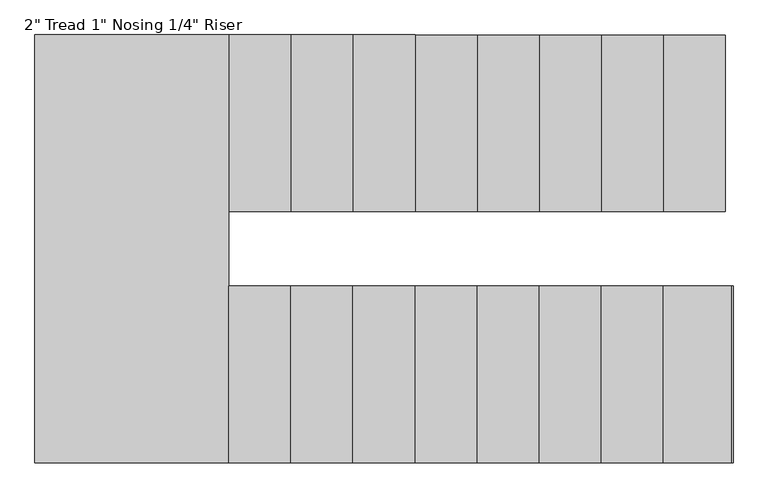
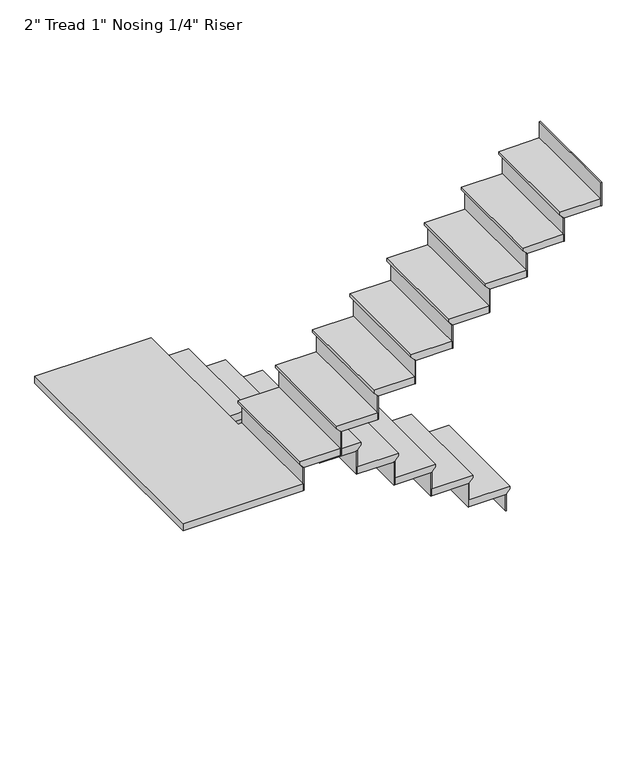
"""IFC4 building model written with IfcOpenShell, lengths in millimetres: stair flight geometry."""

from ifc_helpers import new_model, si_unit, origin, place, context, project, spatial, faceted_brep, source, transform, mapped, element, save


def stair_flight_4533c53f(model_context):
    return source(origin(), model_context, "Body", "Brep", [
        faceted_brep([(-2118.1728655, 1192.5797121, 148.8722222), (-2118.1728655, 1192.5797121, 167.9222222), (-2118.1728655, 468.6797121, 167.9222222), (-2118.1728655, 468.6797121, 148.8722222), (-2143.5728655, 1192.5797121, 123.4722222), (-2143.5728655, 468.6797121, 123.4722222), (-2397.5728655, 1192.5797121, 167.9222222), (-2397.5728655, 468.6797121, 167.9222222), (-2143.5728655, 468.6797121, 117.1222222), (-2397.5728655, 468.6797121, 117.1222222), (-2397.5728655, 1192.5797121, 117.1222222), (-2143.5728655, 1192.5797121, 117.1222222)], [[[0, 1, 2, 3]], [[4, 0, 3, 5]], [[2, 1, 6, 7]], [[8, 9, 10, 11]], [[2, 7, 9, 8, 5, 3]], [[8, 11, 4, 5]], [[6, 1, 0, 4, 11, 10]], [[7, 6, 10, 9]]]),
        faceted_brep([(-2143.5728655, 1192.5797121, 117.1222222), (-2143.5728655, 1192.5797121, 0.0), (-2149.9228655, 1192.5797121, 0.0), (-2149.9228655, 1192.5797121, 117.1222222), (-2143.5728655, 468.6797121, 117.1222222), (-2149.9228655, 468.6797121, 117.1222222), (-2149.9228655, 468.6797121, 0.0), (-2143.5728655, 468.6797121, 0.0)], [[[0, 1, 2, 3]], [[4, 5, 6, 7]], [[1, 0, 4, 7]], [[2, 1, 7, 6]], [[3, 2, 6, 5]], [[0, 3, 5, 4]]]),
        faceted_brep([(-2397.5728655, 1192.5797121, 285.0444444), (-2397.5728655, 1192.5797121, 117.1222222), (-2403.9228655, 1192.5797121, 117.1222222), (-2403.9228655, 1192.5797121, 285.0444444), (-2397.5728655, 468.6797121, 285.0444444), (-2403.9228655, 468.6797121, 285.0444444), (-2403.9228655, 468.6797121, 117.1222222), (-2397.5728655, 468.6797121, 117.1222222)], [[[0, 1, 2, 3]], [[4, 5, 6, 7]], [[1, 0, 4, 7]], [[2, 1, 7, 6]], [[3, 2, 6, 5]], [[0, 3, 5, 4]]]),
        faceted_brep([(-2372.1728655, 468.6797121, 335.8444444), (-2372.1728655, 1192.5797121, 335.8444444), (-2651.5728655, 1192.5797121, 335.8444444), (-2651.5728655, 468.6797121, 335.8444444), (-2397.5728655, 468.6797121, 285.0444444), (-2651.5728655, 468.6797121, 285.0444444), (-2651.5728655, 1192.5797121, 285.0444444), (-2397.5728655, 1192.5797121, 285.0444444), (-2397.5728655, 468.6797121, 291.3944444), (-2372.1728655, 468.6797121, 316.7944444), (-2397.5728655, 1192.5797121, 291.3944444), (-2372.1728655, 1192.5797121, 316.7944444)], [[[0, 1, 2, 3]], [[4, 5, 6, 7]], [[0, 3, 5, 4, 8, 9]], [[4, 7, 10, 8]], [[2, 1, 11, 10, 7, 6]], [[3, 2, 6, 5]], [[11, 1, 0, 9]], [[10, 11, 9, 8]]]),
        faceted_brep([(-2651.5728655, 1192.5797121, 452.9666667), (-2651.5728655, 1192.5797121, 285.0444444), (-2657.9228655, 1192.5797121, 285.0444444), (-2657.9228655, 1192.5797121, 452.9666667), (-2651.5728655, 468.6797121, 452.9666667), (-2657.9228655, 468.6797121, 452.9666667), (-2657.9228655, 468.6797121, 285.0444444), (-2651.5728655, 468.6797121, 285.0444444)], [[[0, 1, 2, 3]], [[4, 5, 6, 7]], [[1, 0, 4, 7]], [[2, 1, 7, 6]], [[3, 2, 6, 5]], [[0, 3, 5, 4]]]),
        faceted_brep([(-2626.1728655, 468.6797121, 503.7666667), (-2626.1728655, 1192.5797121, 503.7666667), (-2905.5728655, 1192.5797121, 503.7666667), (-2905.5728655, 468.6797121, 503.7666667), (-2651.5728655, 468.6797121, 452.9666667), (-2905.5728655, 468.6797121, 452.9666667), (-2905.5728655, 1192.5797121, 452.9666667), (-2651.5728655, 1192.5797121, 452.9666667), (-2651.5728655, 468.6797121, 459.3166667), (-2626.1728655, 468.6797121, 484.7166667), (-2651.5728655, 1192.5797121, 459.3166667), (-2626.1728655, 1192.5797121, 484.7166667)], [[[0, 1, 2, 3]], [[4, 5, 6, 7]], [[0, 3, 5, 4, 8, 9]], [[4, 7, 10, 8]], [[2, 1, 11, 10, 7, 6]], [[3, 2, 6, 5]], [[11, 1, 0, 9]], [[10, 11, 9, 8]]]),
        faceted_brep([(-2905.5728655, 1192.5797121, 620.8888889), (-2905.5728655, 1192.5797121, 452.9666667), (-2911.9228655, 1192.5797121, 452.9666667), (-2911.9228655, 1192.5797121, 620.8888889), (-2905.5728655, 468.6797121, 620.8888889), (-2911.9228655, 468.6797121, 620.8888889), (-2911.9228655, 468.6797121, 452.9666667), (-2905.5728655, 468.6797121, 452.9666667)], [[[0, 1, 2, 3]], [[4, 5, 6, 7]], [[1, 0, 4, 7]], [[2, 1, 7, 6]], [[3, 2, 6, 5]], [[0, 3, 5, 4]]]),
        faceted_brep([(-2880.1728655, 468.6797121, 671.6888889), (-2880.1728655, 1192.5797121, 671.6888889), (-3159.5728655, 1192.5797121, 671.6888889), (-3159.5728655, 468.6797121, 671.6888889), (-2905.5728655, 468.6797121, 620.8888889), (-3159.5728655, 468.6797121, 620.8888889), (-3159.5728655, 1192.5797121, 620.8888889), (-2905.5728655, 1192.5797121, 620.8888889), (-2905.5728655, 468.6797121, 627.2388889), (-2880.1728655, 468.6797121, 652.6388889), (-2905.5728655, 1192.5797121, 627.2388889), (-2880.1728655, 1192.5797121, 652.6388889)], [[[0, 1, 2, 3]], [[4, 5, 6, 7]], [[0, 3, 5, 4, 8, 9]], [[4, 7, 10, 8]], [[2, 1, 11, 10, 7, 6]], [[3, 2, 6, 5]], [[11, 1, 0, 9]], [[10, 11, 9, 8]]]),
        faceted_brep([(-3159.5728655, 1192.5797121, 788.8111111), (-3159.5728655, 1192.5797121, 620.8888889), (-3165.9228655, 1192.5797121, 620.8888889), (-3165.9228655, 1192.5797121, 788.8111111), (-3159.5728655, 468.6797121, 788.8111111), (-3165.9228655, 468.6797121, 788.8111111), (-3165.9228655, 468.6797121, 620.8888889), (-3159.5728655, 468.6797121, 620.8888889)], [[[0, 1, 2, 3]], [[4, 5, 6, 7]], [[1, 0, 4, 7]], [[2, 1, 7, 6]], [[3, 2, 6, 5]], [[0, 3, 5, 4]]]),
        faceted_brep([(-3134.1728655, 468.6797121, 839.6111111), (-3134.1728655, 1192.5797121, 839.6111111), (-3413.5728655, 1192.5797121, 839.6111111), (-3413.5728655, 468.6797121, 839.6111111), (-3159.5728655, 468.6797121, 788.8111111), (-3413.5728655, 468.6797121, 788.8111111), (-3413.5728655, 1192.5797121, 788.8111111), (-3159.5728655, 1192.5797121, 788.8111111), (-3159.5728655, 468.6797121, 795.1611111), (-3134.1728655, 468.6797121, 820.5611111), (-3159.5728655, 1192.5797121, 795.1611111), (-3134.1728655, 1192.5797121, 820.5611111)], [[[0, 1, 2, 3]], [[4, 5, 6, 7]], [[0, 3, 5, 4, 8, 9]], [[4, 7, 10, 8]], [[2, 1, 11, 10, 7, 6]], [[3, 2, 6, 5]], [[11, 1, 0, 9]], [[10, 11, 9, 8]]]),
        faceted_brep([(-3413.5728655, 1192.5797121, 956.7333333), (-3413.5728655, 1192.5797121, 788.8111111), (-3419.9228655, 1192.5797121, 788.8111111), (-3419.9228655, 1192.5797121, 956.7333333), (-3413.5728655, 468.6797121, 956.7333333), (-3419.9228655, 468.6797121, 956.7333333), (-3419.9228655, 468.6797121, 788.8111111), (-3413.5728655, 468.6797121, 788.8111111)], [[[0, 1, 2, 3]], [[4, 5, 6, 7]], [[1, 0, 4, 7]], [[2, 1, 7, 6]], [[3, 2, 6, 5]], [[0, 3, 5, 4]]]),
        faceted_brep([(-3388.1728655, 468.6797121, 1007.5333333), (-3388.1728655, 1192.5797121, 1007.5333333), (-3667.5728655, 1192.5797121, 1007.5333333), (-3667.5728655, 468.6797121, 1007.5333333), (-3413.5728655, 468.6797121, 956.7333333), (-3667.5728655, 468.6797121, 956.7333333), (-3667.5728655, 1192.5797121, 956.7333333), (-3413.5728655, 1192.5797121, 956.7333333), (-3413.5728655, 468.6797121, 963.0833333), (-3388.1728655, 468.6797121, 988.4833333), (-3413.5728655, 1192.5797121, 963.0833333), (-3388.1728655, 1192.5797121, 988.4833333)], [[[0, 1, 2, 3]], [[4, 5, 6, 7]], [[0, 3, 5, 4, 8, 9]], [[4, 7, 10, 8]], [[2, 1, 11, 10, 7, 6]], [[3, 2, 6, 5]], [[11, 1, 0, 9]], [[10, 11, 9, 8]]]),
        faceted_brep([(-3667.5728655, 1192.5797121, 1124.6555556), (-3667.5728655, 1192.5797121, 956.7333333), (-3673.9228655, 1192.5797121, 956.7333333), (-3673.9228655, 1192.5797121, 1124.6555556), (-3667.5728655, 468.6797121, 1124.6555556), (-3673.9228655, 468.6797121, 1124.6555556), (-3673.9228655, 468.6797121, 956.7333333), (-3667.5728655, 468.6797121, 956.7333333)], [[[0, 1, 2, 3]], [[4, 5, 6, 7]], [[1, 0, 4, 7]], [[2, 1, 7, 6]], [[3, 2, 6, 5]], [[0, 3, 5, 4]]]),
        faceted_brep([(-3642.1728655, 468.6797121, 1175.4555556), (-3642.1728655, 1192.5797121, 1175.4555556), (-3921.5728655, 1192.5797121, 1175.4555556), (-3921.5728655, 468.6797121, 1175.4555556), (-3667.5728655, 468.6797121, 1124.6555556), (-3921.5728655, 468.6797121, 1124.6555556), (-3921.5728655, 1192.5797121, 1124.6555556), (-3667.5728655, 1192.5797121, 1124.6555556), (-3667.5728655, 468.6797121, 1131.0055556), (-3642.1728655, 468.6797121, 1156.4055556), (-3667.5728655, 1192.5797121, 1131.0055556), (-3642.1728655, 1192.5797121, 1156.4055556)], [[[0, 1, 2, 3]], [[4, 5, 6, 7]], [[0, 3, 5, 4, 8, 9]], [[4, 7, 10, 8]], [[2, 1, 11, 10, 7, 6]], [[3, 2, 6, 5]], [[11, 1, 0, 9]], [[10, 11, 9, 8]]]),
        faceted_brep([(-3921.5728655, 1192.5797121, 1292.5777778), (-3921.5728655, 1192.5797121, 1124.6555556), (-3927.9228655, 1192.5797121, 1124.6555556), (-3927.9228655, 1192.5797121, 1292.5777778), (-3921.5728655, 468.6797121, 1292.5777778), (-3927.9228655, 468.6797121, 1292.5777778), (-3927.9228655, 468.6797121, 1124.6555556), (-3921.5728655, 468.6797121, 1124.6555556)], [[[0, 1, 2, 3]], [[4, 5, 6, 7]], [[1, 0, 4, 7]], [[2, 1, 7, 6]], [[3, 2, 6, 5]], [[0, 3, 5, 4]]]),
        faceted_brep([(-3896.1728655, 468.6797121, 1343.3777778), (-3896.1728655, 1192.5797121, 1343.3777778), (-4175.5728655, 1192.5797121, 1343.3777778), (-4175.5728655, 468.6797121, 1343.3777778), (-3921.5728655, 468.6797121, 1292.5777778), (-4175.5728655, 468.6797121, 1292.5777778), (-4175.5728655, 1192.5797121, 1292.5777778), (-3921.5728655, 1192.5797121, 1292.5777778), (-3921.5728655, 468.6797121, 1298.9277778), (-3896.1728655, 468.6797121, 1324.3277778), (-3921.5728655, 1192.5797121, 1298.9277778), (-3896.1728655, 1192.5797121, 1324.3277778)], [[[0, 1, 2, 3]], [[4, 5, 6, 7]], [[0, 3, 5, 4, 8, 9]], [[4, 7, 10, 8]], [[2, 1, 11, 10, 7, 6]], [[3, 2, 6, 5]], [[11, 1, 0, 9]], [[10, 11, 9, 8]]]),
        faceted_brep([(-4175.5728655, 1192.5797121, 1460.5), (-4175.5728655, 1192.5797121, 1292.5777778), (-4181.9228655, 1192.5797121, 1292.5777778), (-4181.9228655, 1192.5797121, 1460.5), (-4175.5728655, 468.6797121, 1460.5), (-4181.9228655, 468.6797121, 1460.5), (-4181.9228655, 468.6797121, 1292.5777778), (-4175.5728655, 468.6797121, 1292.5777778)], [[[0, 1, 2, 3]], [[4, 5, 6, 7]], [[1, 0, 4, 7]], [[2, 1, 7, 6]], [[3, 2, 6, 5]], [[0, 3, 5, 4]]]),
        faceted_brep([(-4124.7728655, 163.8797121, 1511.3), (-4150.1728655, 163.8797121, 1511.3), (-4150.1728655, 1192.5797121, 1511.3), (-4943.9394105, 1192.5797121, 1511.3), (-4943.9394105, -560.0202879, 1511.3), (-4124.7728655, -560.0202879, 1511.3), (-4150.1728655, 163.8797121, 1460.5), (-4124.7728655, 163.8797121, 1460.5), (-4124.7728655, -560.0202879, 1460.5), (-4943.9394105, -560.0202879, 1460.5), (-4943.9394105, 1192.5797121, 1460.5), (-4175.5728655, 1192.5797121, 1460.5), (-4175.5728655, 468.6797121, 1460.5), (-4150.1728655, 468.6797121, 1460.5), (-4150.1728655, 468.6797121, 1492.25), (-4150.1728655, 1192.5797121, 1492.25), (-4175.5728655, 468.6797121, 1466.85), (-4175.5728655, 1192.5797121, 1466.85)], [[[0, 1, 2, 3, 4, 5]], [[6, 7, 8, 9, 10, 11, 12, 13]], [[1, 0, 7, 6]], [[2, 1, 6, 13, 14, 15]], [[13, 12, 16, 14]], [[12, 11, 17, 16]], [[3, 2, 15, 17, 11, 10]], [[4, 3, 10, 9]], [[5, 4, 9, 8]], [[0, 5, 8, 7]], [[17, 15, 14, 16]]]),
        faceted_brep([(-4124.7728655, -560.0202879, 1628.4222222), (-4124.7728655, -560.0202879, 1460.5), (-4118.4228655, -560.0202879, 1460.5), (-4118.4228655, -560.0202879, 1628.4222222), (-4124.7728655, 163.8797121, 1628.4222222), (-4118.4228655, 163.8797121, 1628.4222222), (-4118.4228655, 163.8797121, 1460.5), (-4124.7728655, 163.8797121, 1460.5)], [[[0, 1, 2, 3]], [[4, 5, 6, 7]], [[1, 0, 4, 7]], [[2, 1, 7, 6]], [[3, 2, 6, 5]], [[0, 3, 5, 4]]]),
        faceted_brep([(-4150.1728655, 163.8797121, 1679.2222222), (-4150.1728655, -560.0202879, 1679.2222222), (-3870.7728655, -560.0202879, 1679.2222222), (-3870.7728655, 163.8797121, 1679.2222222), (-4124.7728655, 163.8797121, 1628.4222222), (-3870.7728655, 163.8797121, 1628.4222222), (-3870.7728655, -560.0202879, 1628.4222222), (-4124.7728655, -560.0202879, 1628.4222222), (-4124.7728655, 163.8797121, 1634.7722222), (-4150.1728655, 163.8797121, 1660.1722222), (-4124.7728655, -560.0202879, 1634.7722222), (-4150.1728655, -560.0202879, 1660.1722222)], [[[0, 1, 2, 3]], [[4, 5, 6, 7]], [[0, 3, 5, 4, 8, 9]], [[4, 7, 10, 8]], [[2, 1, 11, 10, 7, 6]], [[3, 2, 6, 5]], [[11, 1, 0, 9]], [[10, 11, 9, 8]]]),
        faceted_brep([(-3870.7728655, -560.0202879, 1796.3444444), (-3870.7728655, -560.0202879, 1628.4222222), (-3864.4228655, -560.0202879, 1628.4222222), (-3864.4228655, -560.0202879, 1796.3444444), (-3870.7728655, 163.8797121, 1796.3444444), (-3864.4228655, 163.8797121, 1796.3444444), (-3864.4228655, 163.8797121, 1628.4222222), (-3870.7728655, 163.8797121, 1628.4222222)], [[[0, 1, 2, 3]], [[4, 5, 6, 7]], [[1, 0, 4, 7]], [[2, 1, 7, 6]], [[3, 2, 6, 5]], [[0, 3, 5, 4]]]),
        faceted_brep([(-3896.1728655, 163.8797121, 1847.1444444), (-3896.1728655, -560.0202879, 1847.1444444), (-3616.7728655, -560.0202879, 1847.1444444), (-3616.7728655, 163.8797121, 1847.1444444), (-3870.7728655, 163.8797121, 1796.3444444), (-3616.7728655, 163.8797121, 1796.3444444), (-3616.7728655, -560.0202879, 1796.3444444), (-3870.7728655, -560.0202879, 1796.3444444), (-3870.7728655, 163.8797121, 1802.6944444), (-3896.1728655, 163.8797121, 1828.0944444), (-3870.7728655, -560.0202879, 1802.6944444), (-3896.1728655, -560.0202879, 1828.0944444)], [[[0, 1, 2, 3]], [[4, 5, 6, 7]], [[0, 3, 5, 4, 8, 9]], [[4, 7, 10, 8]], [[2, 1, 11, 10, 7, 6]], [[3, 2, 6, 5]], [[11, 1, 0, 9]], [[10, 11, 9, 8]]]),
        faceted_brep([(-3616.7728655, -560.0202879, 1964.2666667), (-3616.7728655, -560.0202879, 1796.3444444), (-3610.4228655, -560.0202879, 1796.3444444), (-3610.4228655, -560.0202879, 1964.2666667), (-3616.7728655, 163.8797121, 1964.2666667), (-3610.4228655, 163.8797121, 1964.2666667), (-3610.4228655, 163.8797121, 1796.3444444), (-3616.7728655, 163.8797121, 1796.3444444)], [[[0, 1, 2, 3]], [[4, 5, 6, 7]], [[1, 0, 4, 7]], [[2, 1, 7, 6]], [[3, 2, 6, 5]], [[0, 3, 5, 4]]]),
        faceted_brep([(-3642.1728655, 163.8797121, 2015.0666667), (-3642.1728655, -560.0202879, 2015.0666667), (-3362.7728655, -560.0202879, 2015.0666667), (-3362.7728655, 163.8797121, 2015.0666667), (-3616.7728655, 163.8797121, 1964.2666667), (-3362.7728655, 163.8797121, 1964.2666667), (-3362.7728655, -560.0202879, 1964.2666667), (-3616.7728655, -560.0202879, 1964.2666667), (-3616.7728655, 163.8797121, 1970.6166667), (-3642.1728655, 163.8797121, 1996.0166667), (-3616.7728655, -560.0202879, 1970.6166667), (-3642.1728655, -560.0202879, 1996.0166667)], [[[0, 1, 2, 3]], [[4, 5, 6, 7]], [[0, 3, 5, 4, 8, 9]], [[4, 7, 10, 8]], [[2, 1, 11, 10, 7, 6]], [[3, 2, 6, 5]], [[11, 1, 0, 9]], [[10, 11, 9, 8]]]),
        faceted_brep([(-3362.7728655, -560.0202879, 2132.1888889), (-3362.7728655, -560.0202879, 1964.2666667), (-3356.4228655, -560.0202879, 1964.2666667), (-3356.4228655, -560.0202879, 2132.1888889), (-3362.7728655, 163.8797121, 2132.1888889), (-3356.4228655, 163.8797121, 2132.1888889), (-3356.4228655, 163.8797121, 1964.2666667), (-3362.7728655, 163.8797121, 1964.2666667)], [[[0, 1, 2, 3]], [[4, 5, 6, 7]], [[1, 0, 4, 7]], [[2, 1, 7, 6]], [[3, 2, 6, 5]], [[0, 3, 5, 4]]]),
        faceted_brep([(-3388.1728655, 163.8797121, 2182.9888889), (-3388.1728655, -560.0202879, 2182.9888889), (-3108.7728655, -560.0202879, 2182.9888889), (-3108.7728655, 163.8797121, 2182.9888889), (-3362.7728655, 163.8797121, 2132.1888889), (-3108.7728655, 163.8797121, 2132.1888889), (-3108.7728655, -560.0202879, 2132.1888889), (-3362.7728655, -560.0202879, 2132.1888889), (-3362.7728655, 163.8797121, 2138.5388889), (-3388.1728655, 163.8797121, 2163.9388889), (-3362.7728655, -560.0202879, 2138.5388889), (-3388.1728655, -560.0202879, 2163.9388889)], [[[0, 1, 2, 3]], [[4, 5, 6, 7]], [[0, 3, 5, 4, 8, 9]], [[4, 7, 10, 8]], [[2, 1, 11, 10, 7, 6]], [[3, 2, 6, 5]], [[11, 1, 0, 9]], [[10, 11, 9, 8]]]),
        faceted_brep([(-3108.7728655, -560.0202879, 2300.1111111), (-3108.7728655, -560.0202879, 2132.1888889), (-3102.4228655, -560.0202879, 2132.1888889), (-3102.4228655, -560.0202879, 2300.1111111), (-3108.7728655, 163.8797121, 2300.1111111), (-3102.4228655, 163.8797121, 2300.1111111), (-3102.4228655, 163.8797121, 2132.1888889), (-3108.7728655, 163.8797121, 2132.1888889)], [[[0, 1, 2, 3]], [[4, 5, 6, 7]], [[1, 0, 4, 7]], [[2, 1, 7, 6]], [[3, 2, 6, 5]], [[0, 3, 5, 4]]]),
        faceted_brep([(-3134.1728655, 163.8797121, 2350.9111111), (-3134.1728655, -560.0202879, 2350.9111111), (-2854.7728655, -560.0202879, 2350.9111111), (-2854.7728655, 163.8797121, 2350.9111111), (-3108.7728655, 163.8797121, 2300.1111111), (-2854.7728655, 163.8797121, 2300.1111111), (-2854.7728655, -560.0202879, 2300.1111111), (-3108.7728655, -560.0202879, 2300.1111111), (-3108.7728655, 163.8797121, 2306.4611111), (-3134.1728655, 163.8797121, 2331.8611111), (-3108.7728655, -560.0202879, 2306.4611111), (-3134.1728655, -560.0202879, 2331.8611111)], [[[0, 1, 2, 3]], [[4, 5, 6, 7]], [[0, 3, 5, 4, 8, 9]], [[4, 7, 10, 8]], [[2, 1, 11, 10, 7, 6]], [[3, 2, 6, 5]], [[11, 1, 0, 9]], [[10, 11, 9, 8]]]),
        faceted_brep([(-2854.7728655, -560.0202879, 2468.0333333), (-2854.7728655, -560.0202879, 2300.1111111), (-2848.4228655, -560.0202879, 2300.1111111), (-2848.4228655, -560.0202879, 2468.0333333), (-2854.7728655, 163.8797121, 2468.0333333), (-2848.4228655, 163.8797121, 2468.0333333), (-2848.4228655, 163.8797121, 2300.1111111), (-2854.7728655, 163.8797121, 2300.1111111)], [[[0, 1, 2, 3]], [[4, 5, 6, 7]], [[1, 0, 4, 7]], [[2, 1, 7, 6]], [[3, 2, 6, 5]], [[0, 3, 5, 4]]]),
        faceted_brep([(-2880.1728655, 163.8797121, 2518.8333333), (-2880.1728655, -560.0202879, 2518.8333333), (-2600.7728655, -560.0202879, 2518.8333333), (-2600.7728655, 163.8797121, 2518.8333333), (-2854.7728655, 163.8797121, 2468.0333333), (-2600.7728655, 163.8797121, 2468.0333333), (-2600.7728655, -560.0202879, 2468.0333333), (-2854.7728655, -560.0202879, 2468.0333333), (-2854.7728655, 163.8797121, 2474.3833333), (-2880.1728655, 163.8797121, 2499.7833333), (-2854.7728655, -560.0202879, 2474.3833333), (-2880.1728655, -560.0202879, 2499.7833333)], [[[0, 1, 2, 3]], [[4, 5, 6, 7]], [[0, 3, 5, 4, 8, 9]], [[4, 7, 10, 8]], [[2, 1, 11, 10, 7, 6]], [[3, 2, 6, 5]], [[11, 1, 0, 9]], [[10, 11, 9, 8]]]),
        faceted_brep([(-2600.7728655, -560.0202879, 2635.9555556), (-2600.7728655, -560.0202879, 2468.0333333), (-2594.4228655, -560.0202879, 2468.0333333), (-2594.4228655, -560.0202879, 2635.9555556), (-2600.7728655, 163.8797121, 2635.9555556), (-2594.4228655, 163.8797121, 2635.9555556), (-2594.4228655, 163.8797121, 2468.0333333), (-2600.7728655, 163.8797121, 2468.0333333)], [[[0, 1, 2, 3]], [[4, 5, 6, 7]], [[1, 0, 4, 7]], [[2, 1, 7, 6]], [[3, 2, 6, 5]], [[0, 3, 5, 4]]]),
        faceted_brep([(-2626.1728655, 163.8797121, 2686.7555556), (-2626.1728655, -560.0202879, 2686.7555556), (-2346.7728655, -560.0202879, 2686.7555556), (-2346.7728655, 163.8797121, 2686.7555556), (-2600.7728655, 163.8797121, 2635.9555556), (-2346.7728655, 163.8797121, 2635.9555556), (-2346.7728655, -560.0202879, 2635.9555556), (-2600.7728655, -560.0202879, 2635.9555556), (-2600.7728655, 163.8797121, 2642.3055556), (-2626.1728655, 163.8797121, 2667.7055556), (-2600.7728655, -560.0202879, 2642.3055556), (-2626.1728655, -560.0202879, 2667.7055556)], [[[0, 1, 2, 3]], [[4, 5, 6, 7]], [[0, 3, 5, 4, 8, 9]], [[4, 7, 10, 8]], [[2, 1, 11, 10, 7, 6]], [[3, 2, 6, 5]], [[11, 1, 0, 9]], [[10, 11, 9, 8]]]),
        faceted_brep([(-2346.7728655, -560.0202879, 2803.8777778), (-2346.7728655, -560.0202879, 2635.9555556), (-2340.4228655, -560.0202879, 2635.9555556), (-2340.4228655, -560.0202879, 2803.8777778), (-2346.7728655, 163.8797121, 2803.8777778), (-2340.4228655, 163.8797121, 2803.8777778), (-2340.4228655, 163.8797121, 2635.9555556), (-2346.7728655, 163.8797121, 2635.9555556)], [[[0, 1, 2, 3]], [[4, 5, 6, 7]], [[1, 0, 4, 7]], [[2, 1, 7, 6]], [[3, 2, 6, 5]], [[0, 3, 5, 4]]]),
        faceted_brep([(-2092.7728655, -560.0202879, 2971.8), (-2092.7728655, -560.0202879, 2803.8777778), (-2086.4228655, -560.0202879, 2803.8777778), (-2086.4228655, -560.0202879, 2971.8), (-2092.7728655, 163.8797121, 2971.8), (-2086.4228655, 163.8797121, 2971.8), (-2086.4228655, 163.8797121, 2803.8777778), (-2092.7728655, 163.8797121, 2803.8777778)], [[[0, 1, 2, 3]], [[4, 5, 6, 7]], [[1, 0, 4, 7]], [[2, 1, 7, 6]], [[3, 2, 6, 5]], [[0, 3, 5, 4]]]),
        faceted_brep([(-2372.1728655, 163.8797121, 2854.6777778), (-2372.1728655, -560.0202879, 2854.6777778), (-2092.7728655, -560.0202879, 2854.6777778), (-2092.7728655, 163.8797121, 2854.6777778), (-2346.7728655, 163.8797121, 2803.8777778), (-2092.7728655, 163.8797121, 2803.8777778), (-2092.7728655, -560.0202879, 2803.8777778), (-2346.7728655, -560.0202879, 2803.8777778), (-2346.7728655, 163.8797121, 2810.2277778), (-2372.1728655, 163.8797121, 2835.6277778), (-2346.7728655, -560.0202879, 2810.2277778), (-2372.1728655, -560.0202879, 2835.6277778)], [[[0, 1, 2, 3]], [[4, 5, 6, 7]], [[0, 3, 5, 4, 8, 9]], [[4, 7, 10, 8]], [[2, 1, 11, 10, 7, 6]], [[3, 2, 6, 5]], [[11, 1, 0, 9]], [[10, 11, 9, 8]]]),
    ])


if __name__ == "__main__":
    model = new_model("IFC4")
    model_context = context("Model", 3, world=origin())
    ifc_project = project(units=[si_unit("LENGTHUNIT", "METRE", prefix="MILLI")], contexts=[model_context])
    site = spatial("IfcSite", under=ifc_project)
    building = spatial("IfcBuilding", under=site)
    placement = place(None, origin())
    stair_flight_shape = stair_flight_4533c53f(model_context)
    element("IfcStairFlight", 1, ObjectType="2\" Tread 1\" Nosing 1/4\" Riser", at=placement, inside=building, context=model_context, shape_type="MappedRepresentation", body=[
        mapped(stair_flight_shape, transform((0.0, 0.0, 0.0), x_axis=(1.0, 0.0, 0.0), y_axis=(0.0, 1.0, 0.0), z_axis=(0.0, 0.0, 1.0))),
    ])
    save(model, "model.ifc")
